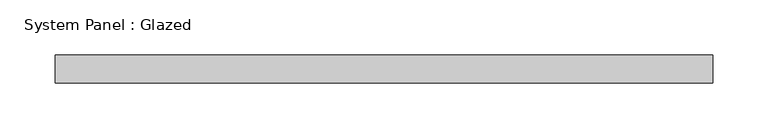
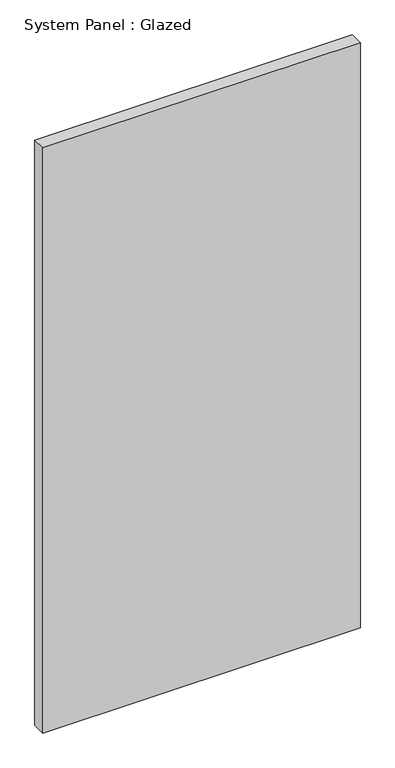
"""IFC4 building model written with IfcOpenShell, lengths in millimetres: plate geometry, System Panel : Glazed."""

from ifc_helpers import new_model, si_unit, origin, origin_with_axes, place, context, project, spatial, polyline, outline, extrude, source, transform, mapped, element, save


def system_panel_glazed_6a84950c(model_context):
    return source(origin(), model_context, "Body", "SweptSolid", [
        extrude(outline(polyline([(298.45, 19.05), (-298.45, 19.05), (-298.45, 44.45), (298.45, 44.45), (298.45, 19.05)])), origin_with_axes(), (0.0, 0.0, 1.0), 1161.9615505),
    ])


if __name__ == "__main__":
    model = new_model("IFC4")
    model_context = context("Model", 3, world=origin())
    ifc_project = project(units=[si_unit("LENGTHUNIT", "METRE", prefix="MILLI")], contexts=[model_context])
    site = spatial("IfcSite", under=ifc_project)
    building = spatial("IfcBuilding", under=site)
    placement = place(None, origin())
    system_panel_glazed_shape = system_panel_glazed_6a84950c(model_context)
    element("IfcPlate", 1, ObjectType="System Panel : Glazed", at=placement, inside=building, context=model_context, shape_type="MappedRepresentation", body=[
        mapped(system_panel_glazed_shape, transform((0.0, 0.0, 0.0), x_axis=(1.0, 0.0, 0.0), y_axis=(0.0, 1.0, 0.0), z_axis=(0.0, 0.0, 1.0))),
    ])
    save(model, "model.ifc")

# Revit data of these elements
# Type "System Panel : Glazed"
#   Construction Type Id = "GSP4R"
#   Analytic Construction = "1/8 in Pilkington single glazing"
#   Visual Light Transmittance = 0.9
#   Solar Heat Gain Coefficient = 0.86
#   Heat Transfer Coefficient (U) = 1.18115 BTU/(h·ft²·°F)
#   Define Thermal Properties by = 1
# Element 1 (IfcPlate, "System Panel : Glazed")
#   Materials on its faces: "Glass"
# Materials
#   "Glass": class "Glass", colour RGB 0 128 192, transparency 0.75, Description = "Soda Lime Glass", Cost = 0
